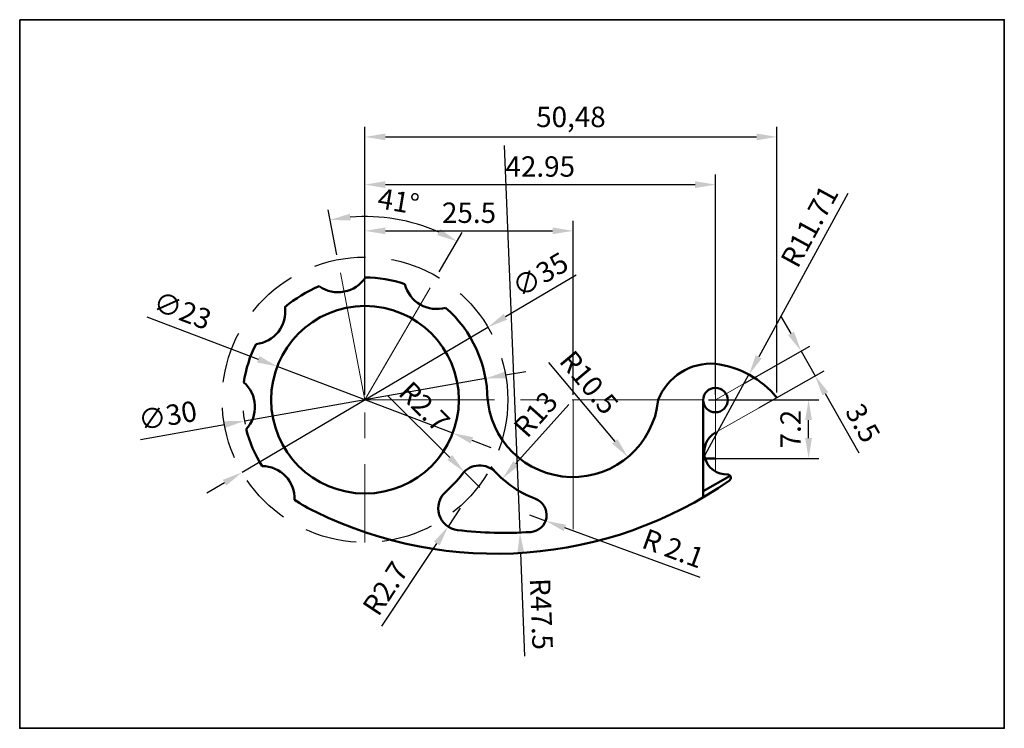
# Model space of a CAD drawing. Units: millimetres. Extents: x 120 to 241, y 102 to 189.
import ezdxf

# ---------------------------------------------------------------- set-up
doc = ezdxf.new("R2010")
doc.units = ezdxf.units.MM
doc.header["$LTSCALE"] = 0.5
doc.linetypes.add('CENTER', pattern=[50.8, 31.75, -6.35, 6.35, -6.35])
doc.linetypes.add('DASHED', pattern=[19.05, 12.7, -6.35])
for name, color, linetype, lineweight in [('M-CNTR', 1, 'CENTER', 18), ('M-DIMS', 2, 'Continuous', 25), ('M-HIDN', 4, 'DASHED', 25), ('M-OUTL', 7, 'Continuous', 50), ('M-TTLB', 7, 'Continuous', 35)]:
    doc.layers.add(name, color=color, linetype=linetype, lineweight=lineweight)
doc.styles.get("Standard").update_dxf_attribs({"font": 'arial.ttf'})
doc.dimstyles.new('ISO-25', dxfattribs={"dimtxt": 2.5, "dimasz": 2.5, "dimexe": 1.25, "dimexo": 0.625, "dimtad": 1, "dimtxsty": 'Standard', "dimcen": 2.5, "dimadec": 0, "dimazin": 0, "dimtfac": 1, "dimtmove": 0, "dimatfit": 3, "dimfxl": 1, "dimarcsym": 0})

# ---------------------------------------------------------------- blocks, each defined once
blk = doc.blocks.new('*D1')
at = {"layer": 'Defpoints', "color": 0, "transparency": 16777216}
for p in [(213.24, 174.84), (162.76, 142.72), (213.24, 142.86)]:
    blk.add_point(p, dxfattribs=at)
at = {"layer": 'M-DIMS', "color": 0, "lineweight": -2, "transparency": 16777216}
for p, q in [((162.76, 143.34), (162.76, 176.09)), ((213.24, 143.49), (213.24, 176.09)), ((165.26, 174.84), (210.74, 174.84))]:
    blk.add_line(p, q, dxfattribs=at)
at = {"layer": 'M-DIMS', "color": 0, "transparency": 16777216}
for points in [[(165.26, 175.26), (165.26, 174.43), (162.76, 174.84)], [(210.74, 175.26), (210.74, 174.43), (213.24, 174.84)]]:
    blk.add_solid(points, dxfattribs=at)
at = {"layer": 'M-DIMS', "color": 0, "transparency": 16777216, "insert": (188, 176.97), "char_height": 2.5, "attachment_point": 5}
blk.add_mtext('50,48', dxfattribs=at)
blk = doc.blocks.new('*D2')
at = {"layer": 'Defpoints', "color": 0, "transparency": 16777216}
for p in [(188.26, 163.32), (162.76, 142.61), (188.26, 142.61)]:
    blk.add_point(p, dxfattribs=at)
at = {"layer": 'M-DIMS', "color": 0, "lineweight": -2, "transparency": 16777216}
for p, q in [((162.76, 143.23), (162.76, 164.57)), ((188.26, 143.23), (188.26, 164.57)), ((165.26, 163.32), (185.76, 163.32))]:
    blk.add_line(p, q, dxfattribs=at)
at = {"layer": 'M-DIMS', "color": 0, "transparency": 16777216}
for points in [[(165.26, 163.74), (165.26, 162.91), (162.76, 163.32)], [(185.76, 163.74), (185.76, 162.91), (188.26, 163.32)]]:
    blk.add_solid(points, dxfattribs=at)
at = {"layer": 'M-DIMS', "color": 0, "transparency": 16777216, "insert": (175.51, 165.22), "char_height": 2.5, "attachment_point": 5}
blk.add_mtext('25.5', dxfattribs=at)
blk = doc.blocks.new('*D3')
at = {"layer": 'Defpoints', "color": 0, "transparency": 16777216}
for p in [(205.71, 168.99), (162.76, 142.61), (205.71, 142.61)]:
    blk.add_point(p, dxfattribs=at)
at = {"layer": 'M-DIMS', "color": 0, "lineweight": -2, "transparency": 16777216}
for p, q in [((162.76, 143.23), (162.76, 170.24)), ((205.71, 143.23), (205.71, 170.24)), ((165.26, 168.99), (203.21, 168.99))]:
    blk.add_line(p, q, dxfattribs=at)
at = {"layer": 'M-DIMS', "color": 0, "transparency": 16777216}
for points in [[(165.26, 169.41), (165.26, 168.57), (162.76, 168.99)], [(203.21, 169.41), (203.21, 168.57), (205.71, 168.99)]]:
    blk.add_solid(points, dxfattribs=at)
at = {"layer": 'M-DIMS', "color": 0, "transparency": 16777216, "insert": (184.24, 170.89), "char_height": 2.5, "attachment_point": 5}
blk.add_mtext('42.95', dxfattribs=at)
blk = doc.blocks.new('*D4')
at = {"layer": 'Defpoints', "color": 0, "transparency": 16777216}
for p in [(217.93, 145.53), (208.75, 144.34), (210.48, 141.3)]:
    blk.add_point(p, dxfattribs=at)
at = {"layer": 'M-DIMS', "color": 0, "lineweight": -2, "transparency": 16777216}
for p, q in [((214.97, 150.74), (213.74, 152.92)), ((209.3, 144.65), (217.29, 149.19)), ((216.21, 148.57), (217.93, 145.53)), ((211.03, 141.6), (219.02, 146.15)), ((219.17, 143.36), (223.28, 136.12))]:
    blk.add_line(p, q, dxfattribs=at)
at = {"layer": 'M-DIMS', "color": 0, "transparency": 16777216}
for points in [[(215.33, 150.95), (214.61, 150.54), (216.21, 148.57)], [(219.53, 143.56), (218.81, 143.15), (217.93, 145.53)]]:
    blk.add_solid(points, dxfattribs=at)
at = {"layer": 'M-DIMS', "color": 0, "transparency": 16777216, "insert": (223.5, 139.59), "char_height": 2.5, "attachment_point": 5, "rotation": 299.6104}
blk.add_mtext('3.5', dxfattribs=at)
blk = doc.blocks.new('*D5')
at = {"layer": 'Defpoints', "color": 0, "transparency": 16777216}
for p in [(209.82, 145.69), (204.21, 135.41)]:
    blk.add_point(p, dxfattribs=at)
at = {"layer": 'M-DIMS', "color": 0, "lineweight": -2, "transparency": 16777216}
for p, q in [((221.95, 167.92), (211.02, 147.88)), ((204.21, 135.41), (209.82, 145.69))]:
    blk.add_line(p, q, dxfattribs=at)
at = {"layer": 'M-DIMS', "color": 0, "transparency": 16777216}
blk.add_solid([(210.65, 148.08), (211.38, 147.68), (209.82, 145.69)], dxfattribs=at)
at = {"layer": 'M-DIMS', "color": 0, "transparency": 16777216, "insert": (217.52, 163.73), "char_height": 2.5, "attachment_point": 5, "rotation": 61.3882}
blk.add_mtext('R11.71', dxfattribs=at)
blk = doc.blocks.new('*D6')
at = {"layer": 'Defpoints', "color": 0, "transparency": 16777216}
for p in [(188.26, 142.61), (179.59, 132.92)]:
    blk.add_point(p, dxfattribs=at)
at = {"layer": 'M-DIMS', "color": 0, "lineweight": -2, "transparency": 16777216}
blk.add_line((187.74, 142.03), (181.25, 134.79), dxfattribs=at)
at = {"layer": 'M-DIMS', "color": 0, "transparency": 16777216}
blk.add_solid([(180.94, 135.06), (181.57, 134.51), (179.59, 132.92)], dxfattribs=at)
at = {"layer": 'M-DIMS', "color": 0, "transparency": 16777216, "insert": (183.92, 140.61), "char_height": 2.5, "attachment_point": 5, "rotation": 48.1439}
blk.add_mtext('R13', dxfattribs=at)
blk = doc.blocks.new('*D7')
at = {"layer": 'Defpoints', "color": 0, "transparency": 16777216}
for p in [(188.24, 143.63), (194.99, 135.58)]:
    blk.add_point(p, dxfattribs=at)
at = {"layer": 'M-DIMS', "color": 0, "lineweight": -2, "transparency": 16777216}
blk.add_line((185.25, 147.19), (193.38, 137.5), dxfattribs=at)
at = {"layer": 'M-DIMS', "color": 0, "transparency": 16777216}
blk.add_solid([(193.7, 137.77), (193.06, 137.23), (194.99, 135.58)], dxfattribs=at)
at = {"layer": 'M-DIMS', "color": 0, "transparency": 16777216, "insert": (189.97, 144.52), "char_height": 2.5, "attachment_point": 5, "rotation": 310.0094}
blk.add_mtext('R10.5', dxfattribs=at)
blk = doc.blocks.new('*D8')
at = {"layer": 'Defpoints', "color": 0, "transparency": 16777216}
for p in [(182.92, 128.48), (184.9, 127.76)]:
    blk.add_point(p, dxfattribs=at)
at = {"layer": 'M-DIMS', "color": 0, "lineweight": -2, "transparency": 16777216}
for p, q in [((182.92, 128.48), (184.9, 127.76)), ((203.85, 120.81), (187.24, 126.9))]:
    blk.add_line(p, q, dxfattribs=at)
at = {"layer": 'M-DIMS', "color": 0, "transparency": 16777216}
blk.add_solid([(187.39, 127.29), (187.1, 126.51), (184.9, 127.76)], dxfattribs=at)
at = {"layer": 'M-DIMS', "color": 0, "transparency": 16777216, "insert": (200.43, 124.07), "char_height": 2.5, "attachment_point": 5, "rotation": 339.8687}
blk.add_mtext('R 2.1', dxfattribs=at)
blk = doc.blocks.new('*D9')
at = {"layer": 'Defpoints', "color": 0, "transparency": 16777216}
for p in [(179.83, 173.78), (181.75, 126.32)]:
    blk.add_point(p, dxfattribs=at)
at = {"layer": 'M-DIMS', "color": 0, "lineweight": -2, "transparency": 16777216}
for p, q in [((179.83, 173.78), (181.75, 126.32)), ((182.36, 111.17), (181.85, 123.82))]:
    blk.add_line(p, q, dxfattribs=at)
at = {"layer": 'M-DIMS', "color": 0, "transparency": 16777216}
blk.add_solid([(182.27, 123.83), (181.43, 123.8), (181.75, 126.32)], dxfattribs=at)
at = {"layer": 'M-DIMS', "color": 0, "transparency": 16777216, "insert": (184.05, 116.32), "char_height": 2.5, "attachment_point": 5, "rotation": 272.3175}
blk.add_mtext('R47.5', dxfattribs=at)
blk = doc.blocks.new('*D10')
at = {"layer": 'Defpoints', "color": 0, "transparency": 16777216}
for p in [(174.91, 133.76), (176.82, 131.85)]:
    blk.add_point(p, dxfattribs=at)
at = {"layer": 'M-DIMS', "color": 0, "lineweight": -2, "transparency": 16777216}
for p, q in [((165.58, 143.09), (173.14, 135.53)), ((176.82, 131.85), (174.91, 133.76))]:
    blk.add_line(p, q, dxfattribs=at)
at = {"layer": 'M-DIMS', "color": 0, "transparency": 16777216}
blk.add_solid([(173.44, 135.83), (172.85, 135.24), (174.91, 133.76)], dxfattribs=at)
at = {"layer": 'M-DIMS', "color": 0, "transparency": 16777216, "insert": (169.81, 141.53), "char_height": 2.5, "attachment_point": 5, "rotation": 315}
blk.add_mtext('R2.7', dxfattribs=at)
blk = doc.blocks.new('*D11')
at = {"layer": 'Defpoints', "color": 0, "transparency": 16777216}
for p in [(174.43, 129.3), (172.94, 127.05)]:
    blk.add_point(p, dxfattribs=at)
at = {"layer": 'M-DIMS', "color": 0, "lineweight": -2, "transparency": 16777216}
for p, q in [((174.43, 129.3), (172.94, 127.05)), ((164.83, 114.84), (171.56, 124.97))]:
    blk.add_line(p, q, dxfattribs=at)
at = {"layer": 'M-DIMS', "color": 0, "transparency": 16777216}
blk.add_solid([(171.21, 125.2), (171.91, 124.74), (172.94, 127.05)], dxfattribs=at)
at = {"layer": 'M-DIMS', "color": 0, "transparency": 16777216, "insert": (165.53, 119.29), "char_height": 2.5, "attachment_point": 5, "rotation": 56.4304}
blk.add_mtext('R2.7', dxfattribs=at)
blk = doc.blocks.new('*D12')
at = {"layer": 'Defpoints', "color": 0, "transparency": 16777216}
for p in [(177.83, 151.51), (147.69, 133.71)]:
    blk.add_point(p, dxfattribs=at)
at = {"layer": 'M-DIMS', "color": 0, "lineweight": -2, "transparency": 16777216}
for p, q in [((188.65, 157.9), (179.98, 152.78)), ((147.69, 133.71), (177.83, 151.51)), ((145.54, 132.43), (143.39, 131.16))]:
    blk.add_line(p, q, dxfattribs=at)
at = {"layer": 'M-DIMS', "color": 0, "transparency": 16777216}
for points in [[(179.77, 153.14), (180.19, 152.42), (177.83, 151.51)], [(145.33, 132.79), (145.75, 132.08), (147.69, 133.71)]]:
    blk.add_solid(points, dxfattribs=at)
at = {"layer": 'M-DIMS', "color": 0, "transparency": 16777216, "insert": (184.39, 157.67), "char_height": 2.5, "attachment_point": 5, "rotation": 30.5723}
blk.add_mtext('∅35', dxfattribs=at)
blk = doc.blocks.new('*D13')
at = {"layer": 'Defpoints', "color": 0, "transparency": 16777216}
for p in [(177.53, 145.21), (147.99, 140)]:
    blk.add_point(p, dxfattribs=at)
at = {"layer": 'M-DIMS', "color": 0, "lineweight": -2, "transparency": 16777216}
for p, q in [((179.99, 145.65), (182.46, 146.08)), ((177.53, 145.21), (147.99, 140)), ((135.25, 137.75), (145.53, 139.57))]:
    blk.add_line(p, q, dxfattribs=at)
blk.add_arc((162.76, 142.61), 15, 185.2303, 191.539, dxfattribs=at)
at = {"layer": 'M-DIMS', "color": 0, "transparency": 16777216}
for points in [[(179.92, 146.06), (180.07, 145.24), (177.53, 145.21)], [(145.45, 139.98), (145.6, 139.16), (147.99, 140)]]:
    blk.add_solid(points, dxfattribs=at)
at = {"layer": 'M-DIMS', "color": 0, "transparency": 16777216, "insert": (138.63, 140.35), "char_height": 2.5, "attachment_point": 5, "rotation": 10.0049}
blk.add_mtext('∅30', dxfattribs=at)
blk = doc.blocks.new('*D14')
at = {"layer": 'Defpoints', "color": 0, "transparency": 16777216}
for p in [(152.01, 146.69), (173.51, 138.52)]:
    blk.add_point(p, dxfattribs=at)
at = {"layer": 'M-DIMS', "color": 0, "lineweight": -2, "transparency": 16777216}
for p, q in [((136.04, 152.76), (149.67, 147.58)), ((173.51, 138.52), (152.01, 146.69)), ((175.85, 137.64), (178.19, 136.75))]:
    blk.add_line(p, q, dxfattribs=at)
at = {"layer": 'M-DIMS', "color": 0, "transparency": 16777216}
for points in [[(149.82, 147.97), (149.53, 147.19), (152.01, 146.69)], [(176, 138.02), (175.7, 137.25), (173.51, 138.52)]]:
    blk.add_solid(points, dxfattribs=at)
at = {"layer": 'M-DIMS', "color": 0, "transparency": 16777216, "insert": (140.27, 153.26), "char_height": 2.5, "attachment_point": 5, "rotation": 339.1977}
blk.add_mtext('∅23', dxfattribs=at)
blk = doc.blocks.new('*D15')
at = {"layer": 'Defpoints', "color": 0, "transparency": 16777216}
for p in [(169.12, 164.16), (159.43, 159.79), (171.55, 157.74), (162.76, 142.61), (162.76, 142.61)]:
    blk.add_point(p, dxfattribs=at)
at = {"layer": 'M-DIMS', "color": 0, "lineweight": -2, "transparency": 16777216}
for p, q in [((159.31, 160.4), (158.25, 165.9)), ((171.86, 158.28), (174.67, 163.12))]:
    blk.add_line(p, q, dxfattribs=at)
blk.add_arc((162.76, 142.61), 22.47, 66.2446, 94.5828, dxfattribs=at)
at = {"layer": 'M-DIMS', "color": 0, "transparency": 16777216}
for points in [[(161.02, 164.59), (160.91, 165.42), (158.49, 164.67)], [(172, 163.55), (171.62, 162.8), (174.04, 162.04)]]:
    blk.add_solid(points, dxfattribs=at)
at = {"layer": 'M-DIMS', "color": 0, "transparency": 16777216, "insert": (166.82, 166.62), "char_height": 2.5, "attachment_point": 5, "rotation": 350.4137}
blk.add_mtext('41°', dxfattribs=at)
blk = doc.blocks.new('*D16')
at = {"layer": 'Defpoints', "color": 0, "transparency": 16777216}
for p in [(204.21, 142.61), (217.12, 142.61), (204.21, 135.41)]:
    blk.add_point(p, dxfattribs=at)
at = {"layer": 'M-DIMS', "color": 0, "lineweight": -2, "transparency": 16777216}
for p, q in [((204.84, 142.61), (218.37, 142.61)), ((217.12, 137.91), (217.12, 140.11)), ((204.84, 135.41), (218.37, 135.41))]:
    blk.add_line(p, q, dxfattribs=at)
at = {"layer": 'M-DIMS', "color": 0, "transparency": 16777216}
for points in [[(216.71, 140.11), (217.54, 140.11), (217.12, 142.61)], [(216.71, 137.91), (217.54, 137.91), (217.12, 135.41)]]:
    blk.add_solid(points, dxfattribs=at)
at = {"layer": 'M-DIMS', "color": 0, "transparency": 16777216, "insert": (215.24, 139.01), "char_height": 2.5, "attachment_point": 5, "rotation": 89.9962}
blk.add_mtext('7.2', dxfattribs=at)

msp = doc.modelspace()

# ---------------------------------------------------------------- linework, layer by layer
at = {"layer": 'M-CNTR'}
for p, q in [((162.761, 142.607), (159.434, 159.788)), ((162.761, 160.107), (162.761, 125.107)), ((162.761, 142.607), (171.546, 157.742)), ((205.711, 149.607), (205.711, 131.593)), ((205.711, 142.607), (211.797, 146.066)), ((162.761, 142.607), (212.79, 142.607)), ((188.261, 142.607), (188.261, 124.79)), ((205.711, 138.584), (213.241, 142.863))]:
    msp.add_line(p, q, dxfattribs=at)
at = {"layer": 'M-HIDN'}
msp.add_circle((162.761, 142.607), 17.5, dxfattribs=at)
at = {"layer": 'M-OUTL'}
for p, q in [((204.211, 142.607), (204.211, 130.688)), ((204.211, 135.407), (205.711, 135.407)), ((204.211, 131.41), (207.525, 133.293))]:
    msp.add_line(p, q, dxfattribs=at)
for centre, radius in [((162.761, 142.607), 11.5), ((205.711, 142.569), 1.5)]:
    msp.add_circle(centre, radius, dxfattribs=at)
for centre, radius, start, end in [((159.462, 159.793), 4, 234.86558, 326.86805), ((162.761, 142.607), 15, 70.9263, 90), ((162.761, 142.607), 15, 111.9263, 130.80734), ((171.546, 157.742), 4, 193.86558, 285.86805), ((148.996, 153.413), 4, 275.86558, 7.86805), ((162.761, 142.607), 15, 0, 48.80734), ((162.761, 142.607), 15, 152.9263, 171.80734), ((205.691, 142.607), 7, 89.83755650756883, 89.83755920681517), ((205.203, 140.039), 7, 85.83903, 158.47792), ((204.211, 135.407), 11.71, 39.54711, 82.64044), ((145.283, 141.732), 4, 316.86558, 48.86805), ((188.241, 143.626), 10.5, 182.2888, 354.43421), ((162.761, 142.607), 15, 193.9263, 212.80734), ((207.069, 136.195), 2.748, 119.61044, 272.51851), ((150.144, 130.48), 4, 357.86558, 89.86805), ((176.821, 131.855), 2.7, 43.22458, 142.59289), ((188.261, 142.607), 13, 219.30765, 249.30096), ((162.761, 142.607), 15, 311.26176, 322.59289), ((207.207, 133.05), 0.4, 304.90665, 92.51851), ((178.824, 173.726), 50, 243.7659, 304.90665), ((162.761, 142.607), 15, 234.9263, 246.25862), ((174.434, 129.302), 2.7, 131.26176, 263.08555), ((182.924, 128.482), 2.1, 273.91059, 69.30096), ((179.828, 173.776), 47.5, 263.08555, 273.91059)]:
    msp.add_arc(centre, radius, start, end, dxfattribs=at)
at = {"layer": 'M-TTLB'}
msp.add_lwpolyline([(120.445, 189.219), (241.108, 189.219), (241.108, 102.316), (120.445, 102.316)], close=True, dxfattribs=at)

# ---------------------------------------------------------------- dimensions: what is measured, and where the dimension line sits
at = {"layer": 'M-DIMS'}
dim = msp.add_linear_dim(base=(213.241, 174.845), p1=(162.761, 142.716), p2=(213.241, 142.863), dimstyle='ISO-25', override={"dimclrd": 0, "dimclre": 0, "dimclrt": 0}, dxfattribs=at)
dim.commit()
dim.dimension.update_dxf_attribs({"geometry": '*D1', "text_midpoint": (188.001, 174.845), "dimtype": 160})
for center, mpoint, text, picture, middle in [((179.828, 173.776), (181.748, 126.315), 'R47.5', '*D9', (184.051, 116.322)), ((176.821, 131.855), (174.912, 133.764), 'R2.7', '*D10', (169.809, 141.526))]:
    dim = msp.add_radius_dim(center=center, mpoint=mpoint, text=text, dimstyle='ISO-25', override={"dimclrd": 0, "dimclre": 0, "dimclrt": 0}, dxfattribs=at)
    dim.commit()
    dim.dimension.update_dxf_attribs({"geometry": picture, "text_midpoint": middle})
for base, p2, text, picture, middle in [((205.711, 168.99), (205.711, 142.607), '42.95', '*D3', (184.236, 170.891)), ((188.261, 163.322), (188.261, 142.607), '25.5', '*D2', (175.511, 165.223))]:
    dim = msp.add_linear_dim(base=base, p1=(162.761, 142.607), p2=p2, text=text, dimstyle='ISO-25', override={"dimclrd": 0, "dimclre": 0, "dimclrt": 0}, dxfattribs=at)
    dim.commit()
    dim.dimension.update_dxf_attribs({"geometry": picture, "text_midpoint": middle})
for center, mpoint, text, picture, middle in [((204.211, 135.407), (209.819, 145.687), 'R11.71', '*D5', (219.172, 162.834)), ((188.241, 143.626), (194.991, 135.583), 'R10.5', '*D7', (188.512, 143.302)), ((174.434, 129.302), (172.941, 127.052), 'R2.7', '*D11', (167.1, 118.25)), ((182.924, 128.482), (184.896, 127.759), 'R 2.1', '*D8', (199.779, 122.304))]:
    dim = msp.add_radius_dim(center=center, mpoint=mpoint, text=text, dimstyle='ISO-25', override={"dimclrd": 0, "dimclre": 0, "dimclrt": 0}, dxfattribs=at)
    dim.commit()
    dim.dimension.update_dxf_attribs({"geometry": picture, "text_midpoint": middle, "dimtype": 164})
dim = msp.add_angular_dim_2l(base=(169.119, 164.16), line1=((162.761, 142.607), (171.546, 157.742)), line2=((162.761, 142.607), (159.434, 159.788)), dimstyle='ISO-25', override={"dimclrd": 0, "dimclre": 0, "dimclrt": 0}, dxfattribs=at)
dim.commit()
dim.dimension.update_dxf_attribs({"geometry": '*D15', "text_midpoint": (166.816, 166.618)})
dim = msp.add_diameter_dim_2p(p1=(147.694, 133.706), p2=(177.828, 151.508), dimstyle='ISO-25', override={"dimclrd": 0, "dimclre": 0, "dimclrt": 0}, dxfattribs=at)
dim.commit()
dim.dimension.update_dxf_attribs({"geometry": '*D12', "text_midpoint": (184.389, 157.674)})
for p1, p2, picture, middle in [((173.511, 138.523), (152.011, 146.691), '*D14', (139.565, 151.42)), ((177.533, 145.213), (147.989, 140.001), '*D13', (138.969, 138.41))]:
    dim = msp.add_diameter_dim_2p(p1=p1, p2=p2, dimstyle='ISO-25', override={"dimclrd": 0, "dimclre": 0, "dimclrt": 0}, dxfattribs=at)
    dim.commit()
    dim.dimension.update_dxf_attribs({"geometry": picture, "text_midpoint": middle, "dimtype": 163})
for p1, p2, distance, text, picture, middle in [((208.754, 144.337), (210.482, 141.296), 8.571, '3.5', '*D4', (223.496, 139.594)), ((204.211, 135.407), (204.212, 142.607), -12.912, '7.2', '*D16', (215.243, 139.007))]:
    dim = msp.add_aligned_dim(p1=p1, p2=p2, distance=distance, text=text, dimstyle='ISO-25', override={"dimclrd": 0, "dimclre": 0, "dimclrt": 0}, dxfattribs=at)
    dim.commit()
    dim.dimension.update_dxf_attribs({"geometry": picture, "text_midpoint": middle})
dim = msp.add_radius_dim(center=(188.261, 142.607), mpoint=(179.587, 132.925), dimstyle='ISO-25', override={"dimclrd": 0, "dimclre": 0, "dimclrt": 0}, dxfattribs=at)
dim.commit()
dim.dimension.update_dxf_attribs({"geometry": '*D6', "text_midpoint": (185.333, 139.339), "dimtype": 164})

doc.saveas('drawing.dxf')
